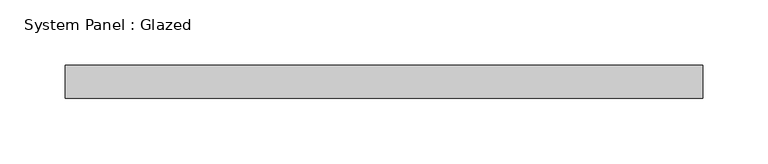
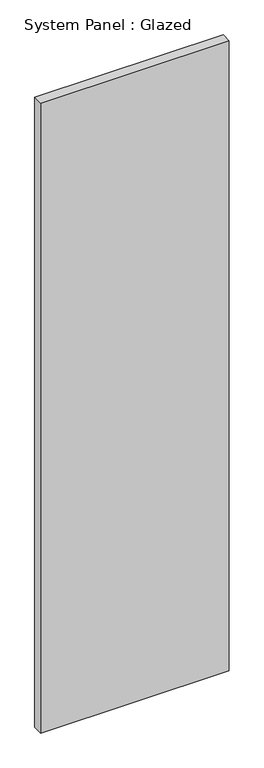
"""IFC4 building model written with IfcOpenShell, lengths in millimetres: plate geometry, System Panel : Glazed."""

from ifc_helpers import new_model, si_unit, origin, origin_with_axes, place, context, project, spatial, polyline, outline, extrude, source, transform, mapped, element, save


def system_panel_glazed_a2b4c657(model_context):
    return source(origin(), model_context, "Body", "SweptSolid", [
        extrude(outline(polyline([(244.475, 19.05), (-244.475, 19.05), (-244.475, 44.45), (244.475, 44.45), (244.475, 19.05)])), origin_with_axes(), (0.0, 0.0, 1.0), 1725.7814546),
    ])


if __name__ == "__main__":
    model = new_model("IFC4")
    model_context = context("Model", 3, world=origin())
    ifc_project = project(units=[si_unit("LENGTHUNIT", "METRE", prefix="MILLI")], contexts=[model_context])
    site = spatial("IfcSite", under=ifc_project)
    building = spatial("IfcBuilding", under=site)
    placement = place(None, origin())
    system_panel_glazed_shape = system_panel_glazed_a2b4c657(model_context)
    element("IfcPlate", 1, ObjectType="System Panel : Glazed", at=placement, inside=building, context=model_context, shape_type="MappedRepresentation", body=[
        mapped(system_panel_glazed_shape, transform((0.0, 0.0, 0.0), x_axis=(1.0, 0.0, 0.0), y_axis=(0.0, 1.0, 0.0), z_axis=(0.0, 0.0, 1.0))),
    ])
    save(model, "model.ifc")

# Revit data of these elements
# Type "System Panel : Glazed"
#   Construction Type Id = "GSP4R"
#   Analytic Construction = "1/8 in Pilkington single glazing"
#   Visual Light Transmittance = 0.9
#   Solar Heat Gain Coefficient = 0.86
#   Heat Transfer Coefficient (U) = 1.18115 BTU/(h·ft²·°F)
#   Define Thermal Properties by = 1
# Element 1 (IfcPlate, "System Panel : Glazed")
#   Materials on its faces: "Glass"
# Materials
#   "Glass": class "Glass", colour RGB 0 128 192, transparency 0.75, Description = "Soda Lime Glass", Cost = 0
